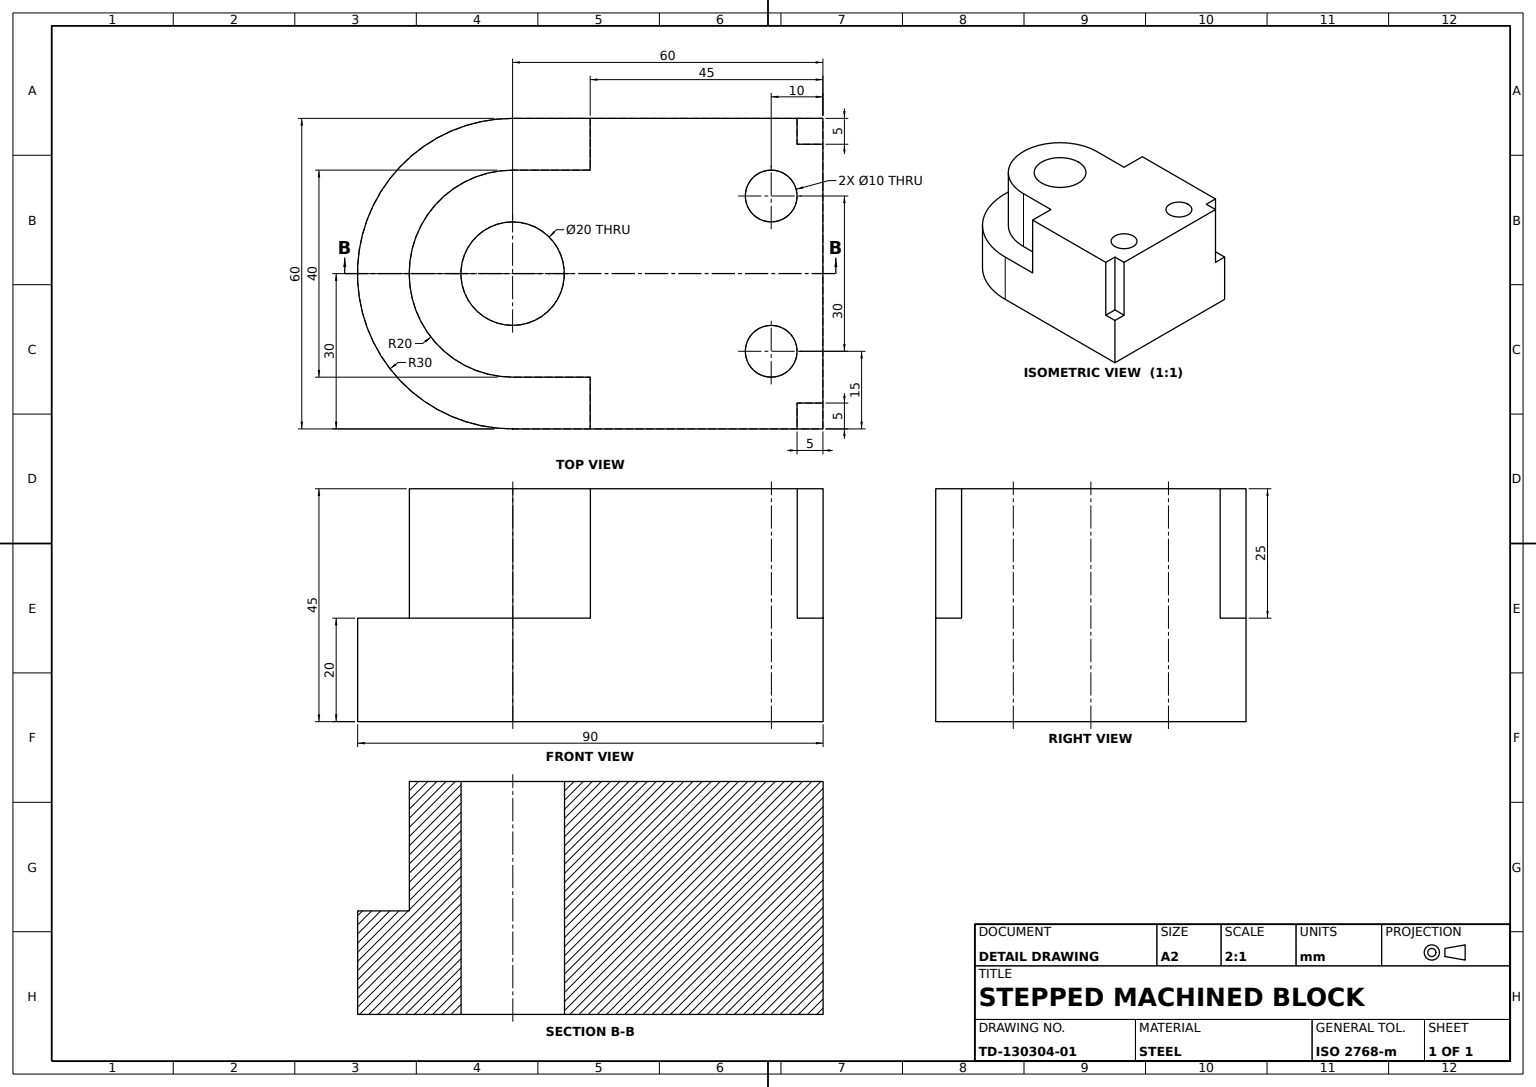
SolidWorks part; units mm, degrees
material "Plain Carbon Steel"
ref_plane "Front Plane" through (0, 0, 0) normal (0, 0, 1) x (1, 0, 0)
ref_plane "Top Plane" through (0, 0, 0) normal (0, 1, 0) x (1, 0, 0)
ref_plane "Right Plane" through (0, 0, 0) normal (1, 0, 0) x (0, 0, -1)
sketch "Base Profile Sketch" plane through (0, 0, 0) normal (0, 1, 0) x (1, 0, 0)
  line L1 (8.3068, 1.3924) -> (8.3068, 31.3924)
  line L2 (8.3068, 1.3924) -> (8.3068, -28.6076)
  line L3 (-51.6932, 31.3924) -> (8.3068, 31.3924)
  line L4 (-51.6932, -28.6076) -> (8.3068, -28.6076)
  arc A1 (-51.6932, 31.3924) -> (-51.6932, -28.6076) centre (-51.6932, 1.3924) ccw
  dimension "D1" = 8.3068
  dimension "D2" = 60
  dimension "D3" = 30
  dimension "D4" = 30
  dimension "D5" = 1.3924
  dimension "D6" = 60
extrude "Base Block" add sketch "Base Profile Sketch" along normal blind 20
sketch "Step Pad 1 Sketch" plane through (0, 20, 0) normal (0, 1, 0) x (1, 0, 0)
  line L1 (8.3068, -28.6076) -> (8.3068, 31.3924) construction
  line L3 (8.3068, -18.6076) -> (8.3068, 21.3924)
  arc A0 (-51.6932, 21.3924) -> (-51.6932, -18.6076) centre (-51.6932, 1.3924) ccw
  circle A1 centre (-51.6932, 1.3924) radius 20
  dimension "D1" = 40
extrude "Step Pad 1" add sketch "Step Pad 1 Sketch" along normal blind 5 contours A0 A1
sketch "Step Pad 2 Sketch" plane through (0, 25, 0) normal (0, 1, 0) x (1, 0, 0)
  line L0 (-51.6932, 21.3924) -> (8.3068, 21.3924)
  line L1 (8.3068, -28.6076) -> (8.3068, 31.3924) construction
  line L2 (8.3068, 21.3924) -> (8.3068, -18.6076)
  line L3 (8.3068, -18.6076) -> (-51.6932, -18.6076)
  circle A0 centre (-51.6932, 1.3924) radius 20 construction
  circle A1 centre (-51.6932, 1.3924) radius 20 construction
  arc A2 (-51.6932, 21.3924) -> (-51.6932, -18.6076) centre (-51.6932, 1.3924) ccw
extrude "Step Pad 2" add sketch "Step Pad 2 Sketch" against normal blind 5
sketch "Round Boss Sketch" plane through (0, 25, 0) normal (0, 1, 0) x (1, 0, 0)
  circle A0 centre (-51.6932, 1.3924) radius 20
  dimension "D1" = 40
extrude "Round Boss" add sketch "Round Boss Sketch" along normal blind 20
sketch "Riser Block 1 Sketch" plane through (0, 25, 0) normal (0, 1, 0) x (1, 0, 0)
  line L0 (-51.6932, 21.3924) -> (8.3068, 21.3924)
  line L1 (8.3068, 21.3924) -> (8.3068, -18.6076)
  line L2 (8.3068, -18.6076) -> (-51.6932, -18.6076)
  line L3 (-51.6932, -18.6076) -> (8.3068, -18.6076) construction
  circle A0 centre (-51.6932, 1.3924) radius 20 construction
  circle A1 centre (-51.6932, 1.3924) radius 20
  arc M1 (-51.6932, 21.3924) -> (-51.6932, -18.6076) centre (-51.6932, 1.3924) cw
  line M2 (-51.6932, -18.6076) -> (8.3068, -18.6076)
  line M3 (8.3068, -18.6076) -> (8.3068, 21.3924)
  line M4 (8.3068, 21.3924) -> (-51.6932, 21.3924)
extrude "Riser Block 1" add sketch "Riser Block 1 Sketch" along normal blind 20 contours M4 M1 M2 M3
sketch "Side Pad 1 Sketch" plane through (0, 20, 0) normal (0, 1, 0) x (1, 0, 0)
  line L0 (8.3068, 21.3924) -> (-51.6932, 21.3924) construction
  line L1 (8.3068, 31.3924) -> (-31.6932, 31.3924)
  line L2 (8.3068, 31.3924) -> (8.3068, 21.3924)
  line L3 (8.3068, 21.3924) -> (-31.6932, 21.3924)
  line L4 (-31.6932, 31.3924) -> (-31.6932, 21.3924)
  dimension "D1" = 40
extrude "Side Pad 1" add sketch "Side Pad 1 Sketch" along normal blind 5
sketch "Riser Block 2 Sketch" plane through (0, 25, 0) normal (0, 1, 0) x (1, 0, 0)
  line L1 (8.3068, 21.3924) -> (-31.6932, 21.3924)
  line L2 (8.3068, 21.3924) -> (8.3068, 31.3924)
  line L3 (8.3068, 31.3924) -> (-31.6932, 31.3924)
  line L4 (-31.6932, 21.3924) -> (-31.6932, 31.3924)
extrude "Riser Block 2" add sketch "Riser Block 2 Sketch" along normal blind 20
sketch "Side Pad 2 Sketch" plane through (0, 20, 0) normal (0, 1, 0) x (1, 0, 0)
  line L0 (-51.6932, -18.6076) -> (8.3068, -18.6076) construction
  line L1 (8.3068, -28.6076) -> (-31.6932, -28.6076)
  line L2 (8.3068, -28.6076) -> (8.3068, -18.6076)
  line L3 (8.3068, -18.6076) -> (-31.6932, -18.6076)
  line L4 (-31.6932, -28.6076) -> (-31.6932, -18.6076)
  dimension "D1" = 40
extrude "Side Pad 2" add sketch "Side Pad 2 Sketch" along normal blind 5
sketch "Riser Block 3 Sketch" plane through (0, 25, 0) normal (0, 1, 0) x (1, 0, 0)
  line L1 (8.3068, -28.6076) -> (-31.6932, -28.6076)
  line L2 (8.3068, -28.6076) -> (8.3068, -18.6076)
  line L3 (8.3068, -18.6076) -> (-31.6932, -18.6076)
  line L4 (-31.6932, -28.6076) -> (-31.6932, -18.6076)
extrude "Riser Block 3" add sketch "Riser Block 3 Sketch" along normal blind 20
sketch "Bore Ø20 Sketch" plane through (0, 45, 0) normal (0, 1, 0) x (1, 0, 0)
  circle A0 centre (-51.6932, 1.3924) radius 10
  dimension "D1" = 20
extrude "Bore Ø20" cut sketch "Bore Ø20 Sketch" against normal blind 76
sketch "Corner Slot 1 Sketch" plane through (0, 45, 0) normal (0, 1, 0) x (1, 0, 0)
  line L0 (8.3068, 31.3924) -> (3.3068, 31.3924)
  line L1 (8.3068, -28.6076) -> (8.3068, 31.3924) construction
  line L2 (8.3068, 31.3924) -> (-31.6932, 31.3924) construction
  line L3 (8.3068, 31.3924) -> (8.3068, 26.3924)
  line L4 (3.3068, 31.3924) -> (3.3068, 26.3924)
  line L5 (8.3068, 26.3924) -> (3.3068, 26.3924)
  dimension "D1" = 5
  dimension "D2" = 5
extrude "Corner Slot 1 5x5" cut sketch "Corner Slot 1 Sketch" against normal blind 25
sketch "Corner Slot 2 Sketch" plane through (0, 45, 0) normal (0, 1, 0) x (1, 0, 0)
  line L0 (8.3068, -28.6076) -> (3.3068, -28.6076)
  line L1 (-31.6932, -28.6076) -> (8.3068, -28.6076) construction
  line L2 (8.3068, -28.6076) -> (8.3068, -23.6076)
  line L3 (8.3068, -28.6076) -> (8.3068, 26.3924) construction
  line L4 (3.3068, -28.6076) -> (3.3068, -23.6076)
  line L5 (8.3068, -23.6076) -> (3.3068, -23.6076)
  dimension "D1" = 5
  dimension "D2" = 5
extrude "Corner Slot 2 5x5" cut sketch "Corner Slot 2 Sketch" against normal blind 25
sketch "Hole 1 Sketch" plane through (0, 45, 0) normal (0, 1, 0) x (1, 0, 0)
  line L0 (-31.6932, 31.3924) -> (-31.6932, 21.3924) construction
  circle A1 centre (-1.6932, -13.6076) radius 5
  dimension "D1" = 10
  dimension "D2" = 30
  dimension "D3" = 45
extrude "Hole 1" cut sketch "Hole 1 Sketch" against normal blind 53 and the other way blind 16
sketch "Hole 2 Sketch" plane through (0, 45, 0) normal (0, 1, 0) x (1, 0, 0)
  line L0 (8.3068, -23.6076) -> (8.3068, 26.3924) construction
  line L1 (3.3068, 26.3924) -> (8.3068, 26.3924) construction
  circle A2 centre (-1.6932, 16.3924) radius 5
  dimension "D1" = 10
  dimension "D2" = 10
  dimension "D3" = 10
extrude "Hole 2" cut sketch "Hole 2 Sketch" against normal blind 122
sketch "Top Block Sketch" plane through (0, 20, 0) normal (0, 1, 0) x (1, 0, 0)
  line L0 (8.3068, 31.3924) -> (-36.6932, 31.3924)
  line L1 (-36.6932, 31.3924) -> (-36.6932, 21.3924)
  line L2 (-31.6932, -28.6076) -> (-36.6932, -28.6076)
  line L3 (-36.6932, -18.6076) -> (-31.6932, -18.6076)
  line L5 (-31.6932, 21.3924) -> (-36.6932, 21.3924)
  line L7 (-36.6932, -18.6076) -> (-36.6932, -28.6076)
  line L8 (-31.6932, -18.6076) -> (-31.6932, -28.6076)
  line L9 (-31.6932, 21.3924) -> (-31.6932, 31.3924)
  line M1 (-51.6932, -28.6076) -> (-31.6932, -28.6076)
  line M2 (-31.6932, -28.6076) -> (-31.6932, -18.6076)
  line M3 (-31.6932, -18.6076) -> (-51.6932, -18.6076)
  line M5 (-51.6932, 21.3924) -> (-31.6932, 21.3924)
  line M6 (-31.6932, 21.3924) -> (-31.6932, 31.3924)
  line M7 (-31.6932, 31.3924) -> (-51.6932, 31.3924)
  dimension "D1" = 45
extrude "Top Block 45" add sketch "Top Block Sketch" along normal up to surface (25 mm away) contours L1 M7 M5 M6 | L7 M3 M1 M2 up to face at (-1.6932, 45, -11.3924)
